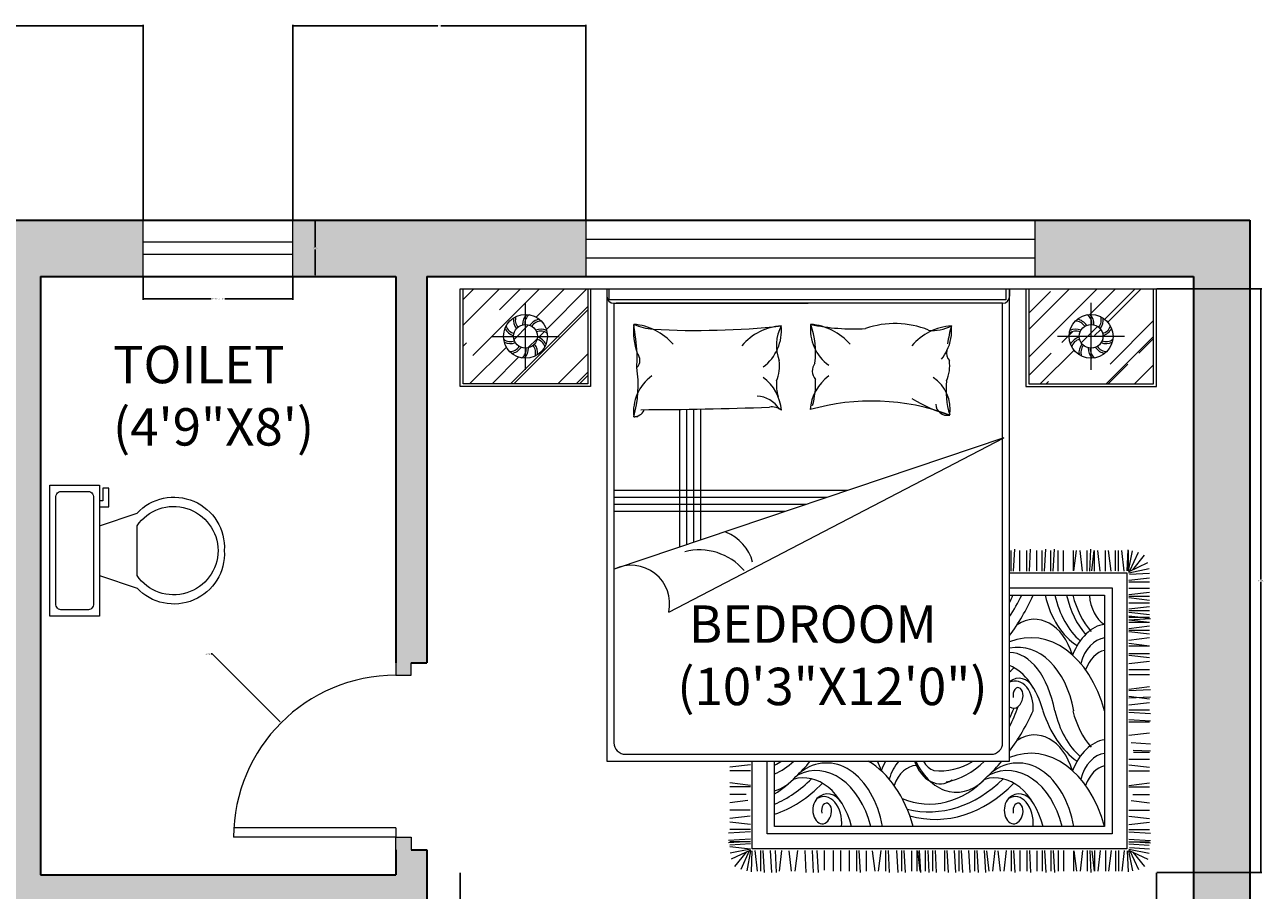
# Model space of a CAD drawing. Units: inches. Extents: x 2948 to 4025, y 2171 to 2966.
# Tile 5 of 6: x 3159 to 3358, y 2670 to 2809. Entities that reach past the tile are written whole.
import ezdxf

# ---------------------------------------------------------------- set-up
doc = ezdxf.new("R2010")
doc.units = ezdxf.units.IN
for name, color, linetype, lineweight in [('A-ANNO-DIMS', 2, 'Continuous', 18), ('A-AREA-IDEN', 7, 'Continuous', 18), ('A-DOOR', 3, 'Continuous', 18), ('A-FLOR-FIXT', 9, 'Continuous', 18), ('A-FURN', 8, 'Continuous', 18), ('A-GLAZ', 4, 'Continuous', 18), ('A-WALL', 7, 'Continuous', 35), ('A-WALL-PATT', 252, 'Continuous', 13)]:
    doc.layers.add(name, color=color, linetype=linetype, lineweight=lineweight)
doc.styles.get("Standard").update_dxf_attribs({"font": 'arial.ttf'})
doc.dimstyles.get("Standard").update_dxf_attribs({"dimtxt": 0.18, "dimasz": 0.18, "dimexe": 0.18, "dimexo": 0.0625, "dimgap": 0.09, "dimtad": 0, "dimtih": 1, "dimtoh": 1, "dimdec": 4, "dimzin": 0, "dimdsep": 46, "dimtxsty": 'Standard', "dimcen": 0.09, "dimadec": 0, "dimazin": 0, "dimtfac": 1, "dimtdec": 4, "dimtofl": 0, "dimtmove": 0, "dimatfit": 3, "dimfxl": 1, "dimtolj": 1, "dimtzin": 0, "dimarcsym": 0})

# ---------------------------------------------------------------- blocks, each defined once
blk = doc.blocks.new('A$C64B41DC1')
for p, q in [((0, 2.5079), (2.9903, 2.5079)), ((0, 2.0879), (0, 2.5079)), ((0.012, 2.4618), (0.0581, 2.5079)), ((0.012, 2.3515), (0.1684, 2.5079)), ((0.012, 2.0999), (0.012, 2.5079)), ((0.0543, 2.2213), (0.3409, 2.5079)), ((0.1689, 2.4179), (0.2589, 2.5079)), ((0.3265, 2.386), (0.4484, 2.5079)), ((0.3699, 2.3332), (0.5445, 2.5079)), ((0.548, 2.5079), (0.548, 2.0999)), ((0.56, 2.5079), (0.56, 2.0879)), ((0.6301, 2.5079), (0.6301, 0.4779)), ((0.6401, 2.461), (0.6401, 2.5079)), ((0.6401, 2.5079), (2.344, 2.5079)), ((2.344, 2.5079), (2.3601, 2.5079)), ((2.344, 2.5079), (2.344, 2.461)), ((2.3601, 2.5079), (2.3601, 2.4761)), ((2.3601, 0.4779), (2.3601, 2.5079)), ((2.4303, 2.5079), (2.4303, 2.0879)), ((2.4423, 2.5079), (2.4423, 2.0999)), ((2.4423, 2.3333), (2.6169, 2.5079)), ((2.4423, 2.2145), (2.7357, 2.5079)), ((2.705, 2.398), (2.8149, 2.5079)), ((2.7691, 2.3772), (2.8998, 2.5079)), ((2.7819, 2.3646), (2.9252, 2.5079)), ((2.9783, 2.0999), (2.9783, 2.5079)), ((2.9903, 2.0879), (2.9903, 2.5079)), ((0.2804, 2.1597), (0.2804, 2.4481)), ((2.344, 2.461), (0.6401, 2.461)), ((2.4423, 2.404), (2.5354, 2.4971)), ((2.7099, 2.1597), (2.7099, 2.4481)), ((0.2157, 2.0999), (0.548, 2.4322)), ((0.2299, 2.0999), (0.548, 2.418)), ((0.6601, 2.4461), (1.4951, 2.4461)), ((0.6601, 2.4461), (0.6601, 0.5579)), ((1.4951, 2.4461), (0.6697, 2.4461)), ((2.3301, 2.4461), (1.4951, 2.4461)), ((2.3301, 0.5579), (2.3301, 2.4461)), ((0.2311, 2.2906), (0.2937, 2.3532)), ((2.6674, 2.2756), (2.7382, 2.3464)), ((2.7914, 2.1846), (2.9783, 2.3715)), ((0.1362, 2.3039), (0.4246, 2.3039)), ((0.2905, 2.2539), (0.3304, 2.2938)), ((0.3405, 2.3039), (0.3605, 2.3238)), ((2.8541, 2.3039), (2.5657, 2.3039)), ((2.5849, 2.2779), (2.6158, 2.3088)), ((2.6158, 2.3088), (2.6313, 2.3243)), ((2.7249, 2.3076), (2.7512, 2.3339)), ((2.7746, 2.0999), (2.9783, 2.3036)), ((2.9144, 2.2312), (2.9783, 2.2951)), ((0.012, 2.261), (0.0275, 2.2765)), ((0.0404, 2.0999), (0.1982, 2.2578)), ((2.4918, 2.0999), (2.6366, 2.2447)), ((0.1365, 2.0999), (0.251, 2.2144)), ((0.4194, 2.0999), (0.548, 2.2285)), ((2.4423, 2.1353), (2.5382, 2.2312)), ((2.7831, 2.0999), (2.8678, 2.1846)), ((2.8962, 2.0999), (2.9783, 2.182)), ((0.4986, 2.0999), (0.548, 2.1493)), ((0.5127, 2.0999), (0.548, 2.1352)), ((0.56, 2.0879), (0, 2.0879)), ((0.548, 2.0999), (0.012, 2.0999)), ((2.4303, 2.0879), (2.9903, 2.0879)), ((2.4423, 2.0999), (2.9783, 2.0999)), ((2.5172, 2.0999), (2.5269, 2.1096)), ((0.9415, 1.9902), (0.9415, 1.3975)), ((0.9715, 1.9906), (0.9715, 1.4076)), ((1.0015, 1.991), (1.0015, 1.4177)), ((1.0315, 1.9916), (1.0315, 1.4279)), ((2.3349, 1.8678), (0.6613, 1.3029)), ((0.8956, 1.1191), (2.3349, 1.8678)), ((1.6636, 1.6412), (0.6601, 1.6412)), ((1.5748, 1.6112), (0.6601, 1.6112)), ((2.3665, 1.295), (2.3665, 1.3839)), ((2.377, 1.295), (2.3822, 1.3891)), ((2.4032, 1.295), (2.4032, 1.3839)), ((2.4346, 1.295), (2.4346, 1.3839)), ((2.4451, 1.295), (2.4503, 1.3891)), ((2.4774, 1.2957), (2.4774, 1.3837)), ((2.5, 1.295), (2.5, 1.3839)), ((2.5105, 1.295), (2.5157, 1.3891)), ((2.5367, 1.295), (2.5367, 1.3839)), ((2.5471, 1.295), (2.5524, 1.3891)), ((2.5681, 1.295), (2.5681, 1.3839)), ((2.5918, 1.295), (2.5918, 1.3839)), ((2.6346, 1.2957), (2.6346, 1.3837)), ((2.6362, 1.2957), (2.6467, 1.3839)), ((2.6729, 1.295), (2.6624, 1.3839)), ((2.6938, 1.295), (2.6938, 1.3839)), ((2.7043, 1.295), (2.7095, 1.3891)), ((2.7127, 1.2957), (2.7232, 1.3839)), ((2.7253, 1.295), (2.7253, 1.3839)), ((2.7494, 1.295), (2.7389, 1.3839)), ((2.7718, 1.295), (2.7718, 1.3839)), ((2.7959, 1.295), (2.7854, 1.3839)), ((2.8146, 1.2957), (2.8146, 1.3837)), ((2.8146, 1.2957), (2.8146, 1.3837)), ((2.8282, 1.295), (2.8282, 1.3839)), ((2.8282, 1.295), (2.8282, 1.3839)), ((2.8523, 1.295), (2.8418, 1.3839)), ((2.8523, 1.295), (2.8418, 1.3839)), ((2.8653, 1.2966), (2.8688, 1.3861)), ((2.8711, 1.2957), (2.8711, 1.3837)), ((2.8711, 1.2957), (2.8875, 1.3822)), ((2.8713, 1.2927), (2.954, 1.3315)), ((2.8765, 1.2958), (2.9132, 1.3758)), ((2.8893, 1.3011), (2.9394, 1.3636)), ((2.3601, 1.2873), (2.8639, 1.2873)), ((2.8639, 1.2873), (2.8639, 0.1018)), ((2.8717, 1.2884), (2.9588, 1.3058)), ((2.8744, 1.2817), (2.9603, 1.2869)), ((2.8716, 1.2565), (2.9605, 1.2669)), ((2.8723, 1.2489), (2.9603, 1.2489)), ((2.3601, 1.2233), (2.7999, 1.2233)), ((2.3601, 1.1913), (2.7679, 1.1912)), ((2.7679, 1.1912), (2.7679, 0.1978)), ((2.7999, 1.2233), (2.7999, 0.1658)), ((2.8716, 1.2212), (2.9605, 1.2212)), ((2.8716, 1.1947), (2.9605, 1.2052)), ((2.8716, 1.181), (2.9605, 1.1705)), ((2.8723, 1.1872), (2.9603, 1.1872)), ((2.8716, 1.1595), (2.9605, 1.1595)), ((2.8716, 1.133), (2.9605, 1.1435)), ((2.8716, 1.1193), (2.9605, 1.1088)), ((2.8723, 1.1255), (2.9603, 1.1255)), ((2.8716, 1.1035), (2.9605, 1.093)), ((2.8716, 1.0965), (2.9605, 1.0965)), ((2.8716, 1.086), (2.9657, 1.0913)), ((2.8716, 1.0756), (2.9605, 1.0756)), ((2.8723, 1.0858), (2.9605, 1.0753)), ((2.8716, 1.0491), (2.9605, 1.0596)), ((2.8716, 1.0354), (2.9605, 1.0249)), ((2.8723, 1.0416), (2.9603, 1.0416)), ((2.8723, 0.9987), (2.9605, 1.0092)), ((2.8723, 0.985), (2.9605, 0.9745)), ((2.8723, 0.9735), (2.9603, 0.9735)), ((2.8716, 0.9346), (2.9605, 0.9241)), ((2.8723, 0.9408), (2.9603, 0.9408)), ((2.8723, 0.8979), (2.9605, 0.9084)), ((2.8723, 0.8726), (2.9603, 0.8726)), ((2.8716, 0.7885), (2.9605, 0.799)), ((2.8723, 0.8505), (2.9603, 0.8505)), ((2.8716, 0.7818), (2.9657, 0.787)), ((2.8716, 0.7503), (2.9657, 0.7556)), ((2.8723, 0.7571), (2.9605, 0.7466)), ((2.8716, 0.7204), (2.9605, 0.7309)), ((2.8716, 0.6995), (2.9605, 0.6995)), ((2.8716, 0.689), (2.9657, 0.6838)), ((2.8716, 0.6576), (2.9657, 0.6523)), ((2.8716, 0.6471), (2.9605, 0.6471)), ((2.8716, 0.5903), (2.9605, 0.6007)), ((2.882, 0.5582), (2.9657, 0.5536)), ((0.7101, 0.5079), (2.2801, 0.5079)), ((2.8716, 0.4877), (2.9603, 0.4877)), ((2.8909, 0.5263), (2.9657, 0.5222)), ((2.8928, 0.5169), (2.9605, 0.5169)), ((0.6301, 0.4779), (2.3601, 0.4779)), ((1.2465, 0.4625), (1.1576, 0.452)), ((1.2465, 0.4365), (1.1577, 0.4365)), ((1.2542, 0.1018), (1.2542, 0.4779)), ((1.3182, 0.1658), (1.3182, 0.4779)), ((1.3502, 0.1978), (1.3502, 0.4779)), ((2.8716, 0.4625), (2.9605, 0.452)), ((2.8716, 0.4365), (2.9603, 0.4365)), ((1.2465, 0.3746), (1.1576, 0.3851)), ((2.8716, 0.3746), (2.9605, 0.3851)), ((1.2465, 0.3684), (1.1577, 0.3684)), ((1.2285, 0.3357), (1.1577, 0.3357)), ((2.8716, 0.3684), (2.9603, 0.3684)), ((2.8896, 0.3357), (2.9603, 0.3357)), ((1.2355, 0.3092), (1.1576, 0.3)), ((1.2457, 0.2676), (1.1577, 0.2676)), ((2.8723, 0.2676), (2.9603, 0.2676)), ((2.8826, 0.3092), (2.9605, 0.3)), ((1.2457, 0.2423), (1.1576, 0.2319)), ((1.2465, 0.2057), (1.1576, 0.2161)), ((2.8716, 0.2057), (2.9605, 0.2161)), ((2.8723, 0.2423), (2.9605, 0.2319)), ((1.2465, 0.1742), (1.1524, 0.169)), ((1.2465, 0.1847), (1.1576, 0.1847)), ((2.7999, 0.1658), (1.3182, 0.1658)), ((2.7679, 0.1978), (1.3502, 0.1978)), ((2.8716, 0.1847), (2.9605, 0.1847)), ((2.8716, 0.1742), (2.9657, 0.169)), ((1.2465, 0.1428), (1.1524, 0.1376)), ((1.2465, 0.1334), (1.1524, 0.1281)), ((1.2465, 0.1323), (1.1576, 0.1323)), ((1.2465, 0.1323), (1.1576, 0.1323)), ((1.2465, 0.1), (1.1576, 0.1105)), ((1.2465, 0.1229), (1.1588, 0.1168)), ((2.8716, 0.1428), (2.9657, 0.1376)), ((2.8716, 0.1334), (2.9657, 0.1281)), ((2.8716, 0.1323), (2.9605, 0.1323)), ((2.8716, 0.1229), (2.9593, 0.1168)), ((2.8744, 0.1074), (2.9603, 0.1022)), ((1.2464, 0.1007), (1.1592, 0.0833)), ((1.2468, 0.0964), (1.1641, 0.0576)), ((1.2288, 0.088), (1.1787, 0.0255)), ((1.2415, 0.0933), (1.2049, 0.0133)), ((1.247, 0.0934), (1.2306, 0.0069)), ((1.2527, 0.0925), (1.2493, 0.003)), ((2.8639, 0.1018), (1.2542, 0.1018)), ((1.2658, 0.0941), (1.2762, 0.0052)), ((1.2899, 0.0941), (1.2899, 0.0052)), ((1.2999, 0.0941), (1.3051, 0)), ((1.3313, 0.0941), (1.3365, 0)), ((1.3523, 0.0941), (1.3575, 0)), ((1.3804, 0.0941), (1.3699, 0.0052)), ((1.4119, 0.0934), (1.4223, 0.0052)), ((1.4485, 0.0941), (1.438, 0.0052)), ((1.48, 0.0941), (1.4852, 0)), ((1.5114, 0.0941), (1.5166, 0)), ((1.5323, 0.0941), (1.5376, 0)), ((1.5638, 0.0941), (1.5638, 0.0105)), ((1.6021, 0.0941), (1.6021, 0.0052)), ((1.6336, 0.0941), (1.6336, 0.0052)), ((1.6702, 0.0941), (1.6702, 0.0052)), ((1.7017, 0.0941), (1.7017, 0.0052)), ((1.7122, 0.0941), (1.7174, 0)), ((1.7445, 0.0934), (1.7445, 0.0054)), ((1.7698, 0.0934), (1.7803, 0.0052)), ((1.8065, 0.0941), (1.796, 0.0052)), ((1.8274, 0.0941), (1.8274, 0.0052)), ((1.8379, 0.0941), (1.8431, 0)), ((1.8746, 0.0941), (1.8798, 0)), ((1.8955, 0.0941), (1.8955, 0.0052)), ((1.906, 0.0941), (1.9113, 0)), ((1.9384, 0.0934), (1.9384, 0.0054)), ((1.9609, 0.0941), (1.9609, 0.0052)), ((1.9636, 0.0934), (1.9741, 0.0052)), ((1.9714, 0.0941), (1.9766, 0)), ((1.9976, 0.0941), (1.9976, 0.0052)), ((2.0081, 0.0941), (2.0133, 0)), ((2.029, 0.0941), (2.029, 0.0052)), ((2.0395, 0.0941), (2.0447, 0)), ((2.0797, 0.0941), (2.0797, 0.0052)), ((2.0902, 0.0941), (2.0954, 0)), ((2.1216, 0.0941), (2.1269, 0)), ((2.1412, 0.0941), (2.1412, 0.0052)), ((2.1517, 0.0941), (2.1569, 0)), ((2.1831, 0.0941), (2.1884, 0)), ((2.2093, 0.0941), (2.2093, 0.0052)), ((2.2198, 0.0941), (2.225, 0)), ((2.2512, 0.0941), (2.2565, 0)), ((2.2603, 0.0934), (2.2707, 0.0052)), ((2.2969, 0.0941), (2.2864, 0.0052)), ((2.3089, 0.0934), (2.3193, 0.0052)), ((2.3455, 0.0941), (2.3351, 0.0052)), ((2.3665, 0.0941), (2.3665, 0.0052)), ((2.377, 0.0941), (2.3822, 0)), ((2.4032, 0.0941), (2.4032, 0.0052)), ((2.4346, 0.0941), (2.4346, 0.0052)), ((2.4451, 0.0941), (2.4503, 0)), ((2.4774, 0.0934), (2.4774, 0.0054)), ((2.5, 0.0941), (2.5, 0.0052)), ((2.5105, 0.0941), (2.5157, 0)), ((2.5367, 0.0941), (2.5367, 0.0052)), ((2.5471, 0.0941), (2.5524, 0)), ((2.5681, 0.0941), (2.5681, 0.0052)), ((2.5918, 0.0941), (2.5918, 0.0052)), ((2.6346, 0.0934), (2.6346, 0.0054)), ((2.6362, 0.0934), (2.6467, 0.0052)), ((2.6729, 0.0941), (2.6624, 0.0052)), ((2.6938, 0.0941), (2.6938, 0.0052)), ((2.7043, 0.0941), (2.7095, 0)), ((2.7127, 0.0934), (2.7232, 0.0052)), ((2.7253, 0.0941), (2.7253, 0.0052)), ((2.7494, 0.0941), (2.7389, 0.0052)), ((2.7718, 0.0941), (2.7718, 0.0052)), ((2.7959, 0.0941), (2.7854, 0.0052)), ((2.8146, 0.0934), (2.8146, 0.0054)), ((2.8282, 0.0941), (2.8282, 0.0052)), ((2.8523, 0.0941), (2.8418, 0.0052)), ((2.8653, 0.0925), (2.8688, 0.003)), ((2.8711, 0.0934), (2.8875, 0.0069)), ((2.8713, 0.0964), (2.954, 0.0576)), ((2.8717, 0.1007), (2.9588, 0.0833)), ((2.8765, 0.0933), (2.9132, 0.0133)), ((2.8893, 0.088), (2.9394, 0.0255))]:
    blk.add_line(p, q)
at = {"ltscale": 10}
for p, q in [((1.4859, 1.5812), (0.6601, 1.5812)), ((1.397, 1.5512), (0.6601, 1.5512))]:
    blk.add_line(p, q, dxfattribs=at)
for centre, radius in [((0.2804, 2.3039), 0.0942), ((2.7099, 2.3039), 0.0942), ((0.2804, 2.3039), 0.051), ((2.7099, 2.3039), 0.051)]:
    blk.add_circle(centre, radius)
for centre, radius, start, end in [((0.6601, 2.4761), 0.03, 180, 270), ((2.3301, 2.4761), 0.03, 270, 0), ((0.3286, 2.3561), 0.0605, 136.17, 182.4897), ((0.3231, 2.3585), 0.0462, 124.3002, 184.538), ((2.6672, 2.3585), 0.0462, 355.462, 55.6998), ((2.6617, 2.3561), 0.0605, 357.5103, 43.83), ((0.2417, 2.3614), 0.0462, 196.3002, 256.538), ((0.2887, 2.3745), 0.0605, 172.17, 218.4897), ((0.2828, 2.3731), 0.0462, 160.3002, 220.538), ((0.3501, 2.3178), 0.0605, 100.17, 146.4897), ((0.347, 2.323), 0.0462, 88.3002, 148.538), ((1.0526, 2.3302), 0.3085, 175.3048, 198.6942), ((-0.8702, 2.0941), 1.6364, 4.8098, 9.1892), ((0.8579, 2.6278), 0.2948, 247.5179, 264.267), ((0.728, 2.111), 0.245, 40.4189, 85.9871), ((1.0164, 5.7096), 3.3803, 266.8134, 276.1602), ((1.3963, 2.1044), 0.245, 94.0129, 139.5811), ((1.1858, 2.3288), 0.1943, 306.5711, 5.89), ((1.5348, 2.2652), 0.1767, 151.7736, 201.6983), ((1.6986, 2.3355), 0.1943, 174.11, 233.4289), ((1.1481, 2.2311), 0.3783, 353.4947, 19.1867), ((1.6871, 3.192), 0.8561, 257.7438, 273.6284), ((1.4882, 2.111), 0.245, 40.4189, 85.9871), ((1.8674, 1.9709), 0.3878, 68.2026, 108.9817), ((2.1269, 2.1044), 0.245, 94.0129, 139.5811), ((2.0342, 2.4856), 0.1563, 261.5958, 298.9092), ((1.9165, 2.3288), 0.1943, 333.7371, 5.89), ((2.6058, 2.2028), 0.517, 163.6046, 172.3273), ((2.6433, 2.323), 0.0462, 31.462, 91.6998), ((2.6402, 2.3178), 0.0605, 33.5103, 79.83), ((2.7075, 2.3731), 0.0462, 319.462, 19.6998), ((2.7016, 2.3745), 0.0605, 321.5103, 7.83), ((2.7486, 2.3614), 0.0462, 283.462, 343.6998), ((0.2153, 2.3276), 0.0462, 232.3002, 292.538), ((0.2457, 2.3659), 0.0605, 208.17, 254.4897), ((0.3449, 2.2742), 0.0605, 64.17, 110.4897), ((0.3455, 2.2802), 0.0462, 52.3002, 112.538), ((0.3191, 2.2464), 0.0462, 16.3002, 76.538), ((0.3151, 2.2419), 0.0605, 28.17, 74.4897), ((2.6448, 2.2802), 0.0462, 67.462, 127.6998), ((2.6454, 2.2742), 0.0605, 69.5103, 115.83), ((2.6752, 2.2419), 0.0605, 105.5103, 151.83), ((2.6712, 2.2464), 0.0462, 103.462, 163.6998), ((2.775, 2.3276), 0.0462, 247.462, 307.6998), ((2.7446, 2.3659), 0.0605, 285.5103, 331.83), ((0.2158, 2.3336), 0.0605, 244.17, 290.4897), ((0.2138, 2.2848), 0.0462, 268.3002, 328.538), ((0.2107, 2.29), 0.0605, 280.17, 326.4897), ((0.2377, 2.2493), 0.0462, 304.3002, 4.538), ((0.2322, 2.2517), 0.0605, 316.17, 2.4897), ((0.2779, 2.2347), 0.0462, 340.3002, 40.538), ((0.272, 2.2333), 0.0605, 352.17, 38.4897), ((1.9165, 2.3288), 0.1943, 320.9404, 333.7371), ((2.1347, 2.2313), 0.0459, 165.3506, 223.2684), ((2.7182, 2.2333), 0.0605, 141.5103, 187.83), ((2.7123, 2.2347), 0.0462, 139.462, 199.6998), ((2.7581, 2.2517), 0.0605, 177.5103, 223.83), ((2.7526, 2.2493), 0.0462, 175.462, 235.6998), ((2.7796, 2.29), 0.0605, 213.5103, 259.83), ((2.7765, 2.2848), 0.0462, 211.462, 271.6998), ((2.7744, 2.3336), 0.0605, 249.5103, 295.83), ((0.7274, 2.2013), 0.0446, 314.4736, 42.1713), ((-1.6008, 2.277), 2.3618, 357.3905, 358.8876), ((1.204, 2.1778), 0.1681, 337.017, 7.5368), ((1.5671, 2.1546), 0.0547, 142.0833, 220.902), ((1.9346, 2.1778), 0.1681, 337.017, 7.5368), ((0.9385, 1.978), 0.1943, 126.5711, 185.89), ((0.2688, 2.0945), 0.4956, 344.0243, 8.7071), ((1.7059, 1.9714), 0.204, 127.1197, 175.09), ((1.1858, 1.9714), 0.1943, 4.3181, 53.4289), ((1.5415, 2.0969), 0.1834, 175.2233, 196.23), ((1.1965, 2.0983), 0.3299, 343.7954, 3.5554), ((1.9394, 1.991), 0.1651, 351.2621, 55.7572), ((2.4617, 2.0719), 0.3745, 173.8296, 196.4356), ((1.2687, 1.9248), 0.1223, 33.628, 86.4744), ((1.7676, 1.0629), 0.9631, 69.6507, 105.9631), ((2.2748, 2.5795), 0.6373, 238.3499, 254.3137), ((0.7417, 2.0149), 0.057, 273.4709, 328.5412), ((0.7246, 18.8439), 16.8552, 270.17399, 272.05214), ((1.3401, 1.9404), 0.0603, 49.0991, 101.3702), ((2.0911, 2.0123), 0.0478, 179.7727, 283.8018), ((0.728, 2.2025), 0.245, 274.0129, 278.3417), ((1.0747, 1.2871), 0.1871, 14.1863, 69.1212), ((1.0274, 1.1334), 0.2527, 40.629, 104.3712), ((0.7347, 1.1553), 0.1649, 347.3109, 116.4454), ((0.7101, 0.5579), 0.05, 180, 270), ((2.2801, 0.5579), 0.05, 270, 0)]:
    blk.add_arc(centre, radius, start, end)
for centre, major_axis, ratio, start_param, end_param in [((1.9938, 1.6262), (0, -0.7531), 0.68, 0.797284, 0.954936), ((2.0643, 1.466), (0, -0.5322), 0.68, 7.239912, 7.311536), ((1.9052, 1.7397), (0, -0.9842), 0.68, 0.74745, 0.979724), ((2.7455, 1.3081), (0, 0.3614), 0.68, 1.900046, 2.742661), ((2.7868, 1.3081), (0, 0.3614), 0.68, 1.900046, 2.614747), ((2.8372, 1.3081), (0, 0.3614), 0.68, 1.900046, 2.479658), ((2.8607, 1.3211), (0, 0.3614), 0.68, 1.938265, 2.479658), ((2.8057, 1.2079), (0, -0.1524), 0.68, 4.821745, 5.895886), ((2.4665, 0.8216), (0, -0.2664), 0.68, 2.006169, 3.565187), ((2.7862, 0.8069), (0, -0.2615), 0.68, 3.244645, 4.205018), ((2.4513, 0.5069), (0, 0.502), 0.68, 5.095327, 6.553458), ((2.396, 0.6032), (0, 0.3641), 0.68, -1.3172, 0.145284), ((2.7784, 0.8289), (0, -0.1802), 0.68, 3.227058, 4.318474), ((2.3507, 0.5642), (0.0073, 0.3819), 0.56205, -1.21172, -0.009991), ((2.7821, 0.7971), (0, -0.1589), 0.68, 3.272942, 4.229533), ((2.2964, 0.5771), (0, -0.3263), 0.68, 1.938944, 2.850232), ((2.0403, 1.6015), (0, -0.8763), 0.68, 6.849801, 6.887077), ((2.4005, 0.7132), (0, -0.1214), 0.68, 2.284368, 3.652258), ((2.3834, 0.7081), (0, 0.1147), 0.68, 4.593909, 6.585576), ((2.3774, 0.7653), (0, -0.0593), 0.68, 5.841311, 7.755362), ((2.3961, 0.7628), (0, -0.0317), 0.68, 1.462497, 5.046281), ((1.9938, 1.1295), (-0.0678, 0.7439), 0.610498, 3.917146, 4.063997), ((2.0643, 0.9693), (0, -0.5322), 0.68, 7.239912, 7.336618), ((1.9052, 1.243), (0, -0.9842), 0.68, 0.74745, 0.979724), ((2.7455, 0.8114), (-0.0599, 0.3735), 0.695517, 1.775813, 2.548612), ((2.7868, 0.8114), (0, 0.3614), 0.68, 1.900046, 2.614747), ((2.8607, 0.8243), (0, 0.3614), 0.68, 1.938265, 2.479658), ((2.4665, 0.3249), (0, -0.2664), 0.68, 2.006169, 3.565187), ((2.4513, 0.0102), (0, 0.502), 0.68, 5.095327, 6.553458), ((2.7862, 0.3102), (0, -0.2615), 0.68, 3.244645, 4.205018), ((1.5283, 0.0674), (0, -0.3703), 0.68, 1.930561, 3.464283), ((1.5736, 0.1065), (0, 0.3641), 0.68, -1.3172, 0.476403), ((2.3507, 0.0674), (0, -0.3703), 0.68, 1.930561, 3.464283), ((2.396, 0.1065), (0, 0.3641), 0.68, -1.3172, 0.476403), ((2.7784, 0.3322), (0, -0.1802), 0.68, 3.227058, 4.318474), ((1.242, 0.9693), (0, -0.5322), 0.68, 6.586764, 6.677612), ((1.1714, 1.1295), (-0.1157, 0.7241), 0.59432, 3.291697, 3.50733), ((1.474, 0.0804), (0, -0.3263), 0.68, 1.938944, 3.339184), ((1.0828, 1.243), (0, -0.9842), 0.68, 0.565948, 0.680366), ((1.6289, 0.0102), (0, 0.502), 0.68, 6.655152, 6.661293), ((1.6289, 0.0102), (0, 0.502), 0.68, 5.095327, 5.911219), ((1.6442, 0.3249), (0, -0.2664), 0.68, 2.006169, 2.182797), ((1.9638, 0.3102), (0, -0.2615), 0.68, 4.015924, 4.205018), ((1.956, 0.3322), (0, -0.1802), 0.68, 3.770744, 4.318474), ((1.9597, 0.3004), (0, -0.1589), 0.68, 3.14258, 4.229533), ((2.0606, 0.5616), (0, -0.1803), 0.68, 5.194792, 5.929328), ((2.0606, 0.5616), (0, -0.1803), 0.68, 5.194792, 6.723255), ((2.1315, 0.6603), (0, -0.3155), 0.68, 5.328638, 6.949396), ((2.0549, 0.5656), (0, -0.1303), 0.68, 5.450951, 6.054641), ((2.0643, 0.9693), (0, -0.5322), 0.68, 6.20013, 6.677612), ((1.9938, 1.1295), (-0.0678, 0.7439), 0.610498, 3.199135, 3.592282), ((2.2964, 0.0804), (0, -0.3263), 0.68, 1.938944, 3.339184), ((1.9052, 1.243), (0, -0.9842), 0.68, 0.565948, 0.680366), ((2.4513, 0.0102), (0, 0.502), 0.68, 6.655152, 6.661293), ((2.7821, 0.3004), (0, -0.1589), 0.68, 3.272942, 4.229533), ((1.1933, 0.9181), (0, -0.624), 0.68, 0.378672, 0.625379), ((1.3091, 0.6603), (0, -0.3155), 0.68, 6.475719, 6.949396), ((1.1911, 1.1066), (0, 0.8458), 0.68, 3.421828, 3.728616), ((1.2179, 1.1047), (0, -0.8763), 0.68, 6.507006, 6.887077), ((2.0157, 0.9181), (0, -0.624), 0.68, -0.280078, 0.625379), ((2.0135, 1.1066), (0, 0.8458), 0.68, 2.978727, 3.728616), ((2.0403, 1.1047), (0, -0.8763), 0.68, 6.099302, 6.887077), ((1.5781, 0.2165), (0, -0.1214), 0.68, 2.284368, 3.726131), ((1.561, 0.2114), (0, 0.1147), 0.68, 4.593909, 6.647252), ((2.4005, 0.2165), (0, -0.1214), 0.68, 2.284368, 3.726131), ((2.3834, 0.2114), (0, 0.1147), 0.68, 4.593909, 6.647252), ((1.555, 0.2685), (0, -0.0593), 0.68, 3.732151, 7.755362), ((1.5737, 0.2661), (0, -0.0317), 0.68, 1.462497, 5.046281), ((2.3774, 0.2685), (0, -0.0593), 0.68, 3.732151, 7.755362), ((2.3961, 0.2661), (0, -0.0317), 0.68, 1.462497, 5.046281)]:
    blk.add_ellipse(centre, major_axis=major_axis, ratio=ratio, start_param=start_param, end_param=end_param)
blk = doc.blocks.new('*U8')
for p, q in [((9.5, -6), (9.5, -2)), ((-10, -8.5), (-8, -8.5)), ((-10, -9.5), (-10, -8.5)), ((-7, -9.5), (-10, -9.5)), ((-8, -8.5), (-8, -8)), ((-7, -8), (-7, -9.5)), ((-4, -8), (-6, -14)), ((4, -8), (6, -14)), ((4, -14), (-4, -14))]:
    blk.add_line(p, q)
blk.add_lwpolyline([(10.5, -8), (10.5, 0), (-10.5, 0), (-10.5, -8)], close=True)
for points in [[(8.5, -1), (-8.5, -1)], [(-9.5, -2), (-9.5, -6)], [(-8.5, -7), (8.5, -7)]]:
    blk.add_lwpolyline(points)
for centre, radius, start, end in [((-8.625, -1.875), 0.8839, 81.8699, 188.1301), ((8.625, -1.875), 0.8839, 351.8699, 98.1301), ((-8.625, -6.125), 0.8839, 171.869898, 278.1301), ((8.625, -6.125), 0.8839, 261.8699, 8.1301), ((-0.4772, -19.9188), 8.0953, 133.01722, 273.38), ((0.0374, -19.8731), 7.127, 124.50543, 269.7), ((-0.0373, -19.8731), 7.127, 270.3, 55.4946), ((0.4773, -19.9188), 8.0953, 266.62, 46.9828)]:
    blk.add_arc(centre, radius, start, end)
blk = doc.blocks.new('DOOR-SWING-26IN')
for p, q in [((26, 30), (26, 28)), ((28.5, 28), (28.5, 30)), ((26, 28), (28.5, 28)), ((26, 2), (0, 2)), ((26, 3.5), (0.04, 3.5)), ((26, 3.5), (26, 2)), ((26, 0), (26, 2)), ((26, 2), (28.5, 2)), ((28.5, 2), (28.5, 0))]:
    blk.add_line(p, q)
blk.add_arc((26, 2), 26, 90, 180)
blk = doc.blocks.new('WIN-72IN')
for p, q in [((0, 0), (0, 9)), ((72, 0), (72, 9)), ((72, 6), (0, 6)), ((72, 3), (0, 3))]:
    blk.add_line(p, q)
blk = doc.blocks.new('WIN-24IN')
for p, q in [((0, 0), (0, 9)), ((24, 0), (24, 9)), ((24, 5.5), (0, 5.5)), ((24, 3.5), (0, 3.5))]:
    blk.add_line(p, q)
blk = doc.blocks.new('*D23')
at = {"layer": 'A-ANNO-DIMS', "color": 0, "lineweight": -2, "transparency": 16777216}
for p, q in [((3178.01, 2768.92), (3178.01, 2765.21)), ((3202.01, 2768.92), (3202.01, 2765.21)), ((3178.19, 2765.39), (3188.9, 2765.39)), ((3201.83, 2765.39), (3191.13, 2765.39))]:
    blk.add_line(p, q, dxfattribs=at)
at = {"layer": 'A-ANNO-DIMS', "color": 0, "transparency": 16777216}
for points in [[(3178.19, 2765.42), (3178.19, 2765.36), (3178.01, 2765.39)], [(3201.83, 2765.42), (3201.83, 2765.36), (3202.01, 2765.39)]]:
    blk.add_solid(points, dxfattribs=at)
at = {"layer": 'Defpoints', "color": 0, "transparency": 16777216}
for p in [(3178.01, 2768.99), (3202.01, 2768.99), (3202.01, 2765.39)]:
    blk.add_point(p, dxfattribs=at)
at = {"layer": 'A-ANNO-DIMS', "color": 0, "transparency": 16777216, "insert": (3190.01, 2765.39), "char_height": 0.18, "attachment_point": 5}
blk.add_mtext('\\A1;WINDOW 24 TYP.', dxfattribs=at)
blk = doc.blocks.new('*D24')
at = {"layer": 'A-ANNO-DIMS', "color": 0, "lineweight": -2, "transparency": 16777216}
for p, q in [((3202.08, 2777.99), (3205.79, 2777.99)), ((3205.61, 2777.81), (3205.61, 2773.67)), ((3205.61, 2769.17), (3205.61, 2773.3)), ((3202.08, 2768.99), (3205.79, 2768.99))]:
    blk.add_line(p, q, dxfattribs=at)
at = {"layer": 'A-ANNO-DIMS', "color": 0, "transparency": 16777216}
for points in [[(3205.58, 2777.81), (3205.64, 2777.81), (3205.61, 2777.99)], [(3205.58, 2769.17), (3205.64, 2769.17), (3205.61, 2768.99)]]:
    blk.add_solid(points, dxfattribs=at)
at = {"layer": 'Defpoints', "color": 0, "transparency": 16777216}
for p in [(3202.01, 2777.99), (3205.61, 2777.99), (3202.01, 2768.99)]:
    blk.add_point(p, dxfattribs=at)
at = {"layer": 'A-ANNO-DIMS', "color": 0, "transparency": 16777216, "insert": (3205.61, 2773.49), "char_height": 0.18, "attachment_point": 5}
blk.add_mtext('\\A1;9 TYP.', dxfattribs=at)
blk = doc.blocks.new('*D27')
at = {"layer": 'A-ANNO-DIMS', "color": 0, "lineweight": -2, "transparency": 16777216}
for p, q in [((3228.87, 2673.27), (3228.87, 2656.41)), ((3340.53, 2673.27), (3340.53, 2656.41)), ((3229.05, 2656.59), (3283.31, 2656.59)), ((3340.35, 2656.59), (3286.08, 2656.59))]:
    blk.add_line(p, q, dxfattribs=at)
at = {"layer": 'A-ANNO-DIMS', "color": 0, "transparency": 16777216}
for points in [[(3229.05, 2656.62), (3229.05, 2656.56), (3228.87, 2656.59)], [(3340.35, 2656.62), (3340.35, 2656.56), (3340.53, 2656.59)]]:
    blk.add_solid(points, dxfattribs=at)
at = {"layer": 'Defpoints', "color": 0, "transparency": 16777216}
for p in [(3228.87, 2673.34), (3340.53, 2673.34), (3340.53, 2656.59)]:
    blk.add_point(p, dxfattribs=at)
at = {"layer": 'A-ANNO-DIMS', "color": 0, "transparency": 16777216, "insert": (3284.7, 2656.59), "char_height": 0.18, "attachment_point": 5}
blk.add_mtext('\\A1;BED GROUP 112 TYP.', dxfattribs=at)
blk = doc.blocks.new('*D28')
at = {"layer": 'A-ANNO-DIMS', "color": 0, "lineweight": -2, "transparency": 16777216}
for p, q in [((3340.59, 2766.99), (3357.46, 2766.99)), ((3357.28, 2766.81), (3357.28, 2720.34)), ((3357.28, 2673.52), (3357.28, 2719.98)), ((3340.59, 2673.34), (3357.46, 2673.34))]:
    blk.add_line(p, q, dxfattribs=at)
at = {"layer": 'A-ANNO-DIMS', "color": 0, "transparency": 16777216}
for points in [[(3357.25, 2766.81), (3357.31, 2766.81), (3357.28, 2766.99)], [(3357.25, 2673.52), (3357.31, 2673.52), (3357.28, 2673.34)]]:
    blk.add_solid(points, dxfattribs=at)
at = {"layer": 'Defpoints', "color": 0, "transparency": 16777216}
for p in [(3340.53, 2766.99), (3357.28, 2766.99), (3340.53, 2673.34)]:
    blk.add_point(p, dxfattribs=at)
at = {"layer": 'A-ANNO-DIMS', "color": 0, "transparency": 16777216, "insert": (3357.28, 2720.16), "char_height": 0.18, "attachment_point": 5}
blk.add_mtext('\\A1;94 TYP.', dxfattribs=at)
blk = doc.blocks.new('*D38')
at = {"layer": 'A-ANNO-DIMS', "color": 0, "lineweight": -2, "transparency": 16777216}
for p, q in [((2979.45, 2777.99), (2948.13, 2777.99)), ((2948.31, 2777.81), (2948.31, 2507.17)), ((2948.31, 2236.17), (2948.31, 2506.8)), ((3217.45, 2235.99), (2948.13, 2235.99))]:
    blk.add_line(p, q, dxfattribs=at)
at = {"layer": 'A-ANNO-DIMS', "color": 0, "transparency": 16777216}
for points in [[(2948.28, 2777.81), (2948.34, 2777.81), (2948.31, 2777.99)], [(2948.28, 2236.17), (2948.34, 2236.17), (2948.31, 2235.99)]]:
    blk.add_solid(points, dxfattribs=at)
at = {"layer": 'Defpoints', "color": 0, "transparency": 16777216}
for p in [(2948.31, 2777.99), (2979.51, 2777.99), (3217.51, 2235.99)]:
    blk.add_point(p, dxfattribs=at)
at = {"layer": 'A-ANNO-DIMS', "color": 0, "transparency": 16777216, "insert": (2948.31, 2506.99), "char_height": 0.18, "attachment_point": 5}
blk.add_mtext('\\A1;542', dxfattribs=at)
blk = doc.blocks.new('*D40')
at = {"layer": 'A-ANNO-DIMS', "color": 0, "lineweight": -2, "transparency": 16777216}
for p, q in [((3108.51, 2778.05), (3108.51, 2809.37)), ((3108.69, 2809.19), (3142.94, 2809.19)), ((3177.83, 2809.19), (3143.59, 2809.19)), ((3178.01, 2778.05), (3178.01, 2809.37))]:
    blk.add_line(p, q, dxfattribs=at)
at = {"layer": 'A-ANNO-DIMS', "color": 0, "transparency": 16777216}
for points in [[(3108.69, 2809.22), (3108.69, 2809.16), (3108.51, 2809.19)], [(3177.83, 2809.22), (3177.83, 2809.16), (3178.01, 2809.19)]]:
    blk.add_solid(points, dxfattribs=at)
at = {"layer": 'Defpoints', "color": 0, "transparency": 16777216}
for p in [(3178.01, 2809.19), (3108.51, 2777.99), (3178.01, 2777.99)]:
    blk.add_point(p, dxfattribs=at)
at = {"layer": 'A-ANNO-DIMS', "color": 0, "transparency": 16777216, "insert": (3143.26, 2809.19), "char_height": 0.18, "attachment_point": 5}
blk.add_mtext('\\A1;69.5', dxfattribs=at)
blk = doc.blocks.new('*D41')
at = {"layer": 'A-ANNO-DIMS', "color": 0, "lineweight": -2, "transparency": 16777216}
for p, q in [((3202.01, 2778.05), (3202.01, 2809.37)), ((3202.19, 2809.19), (3225.29, 2809.19)), ((3248.83, 2809.19), (3225.74, 2809.19)), ((3249.01, 2778.05), (3249.01, 2809.37))]:
    blk.add_line(p, q, dxfattribs=at)
at = {"layer": 'A-ANNO-DIMS', "color": 0, "transparency": 16777216}
for points in [[(3202.19, 2809.22), (3202.19, 2809.16), (3202.01, 2809.19)], [(3248.83, 2809.22), (3248.83, 2809.16), (3249.01, 2809.19)]]:
    blk.add_solid(points, dxfattribs=at)
at = {"layer": 'Defpoints', "color": 0, "transparency": 16777216}
for p in [(3249.01, 2809.19), (3202.01, 2777.99), (3249.01, 2777.99)]:
    blk.add_point(p, dxfattribs=at)
at = {"layer": 'A-ANNO-DIMS', "color": 0, "transparency": 16777216, "insert": (3225.51, 2809.19), "char_height": 0.18, "attachment_point": 5}
blk.add_mtext('\\A1;47', dxfattribs=at)
blk = doc.blocks.new('*D69')
at = {"layer": 'A-ANNO-DIMS', "color": 0, "lineweight": -2, "transparency": 16777216}
for p, q in [((3188.92, 2708.4), (3189.1, 2708.4)), ((3189.1, 2708.4), (3200, 2697.5)), ((3218.42, 2678.99), (3218.6, 2678.99)), ((3218.51, 2678.9), (3218.51, 2679.08))]:
    blk.add_line(p, q, dxfattribs=at)
at = {"layer": 'A-ANNO-DIMS', "color": 0, "transparency": 16777216}
blk.add_solid([(3200.02, 2697.52), (3199.98, 2697.48), (3200.13, 2697.37)], dxfattribs=at)
at = {"layer": 'Defpoints', "color": 0, "transparency": 16777216}
for p in [(3200.13, 2697.37), (3218.51, 2678.99)]:
    blk.add_point(p, dxfattribs=at)
at = {"layer": 'A-ANNO-DIMS', "color": 0, "transparency": 16777216, "insert": (3188.42, 2708.4), "char_height": 0.18, "attachment_point": 5}
blk.add_mtext('\\A1;2X R26', dxfattribs=at)

msp = doc.modelspace()

# ---------------------------------------------------------------- hatches: boundary and pattern name
at = {"layer": 'A-WALL-PATT'}
h = msp.add_hatch(color=256, dxfattribs=at)
h.dxf.hatch_style = 1
h.paths.add_polyline_path([(3178.0136, 2777.9862), (3108.5136, 2777.9862), (3108.5136, 2768.9862), (3156.5136, 2768.9862), (3156.5136, 2624.9862), (3132.5136, 2624.9862), (3130.5136, 2624.9862), (3130.5136, 2622.4862), (3132.5136, 2622.4862), (3132.5136, 2619.9862), (3161.5136, 2619.9862), (3161.5136, 2667.9862), (3218.5136, 2667.9862), (3218.5136, 2660.9862), (3218.5136, 2658.9862), (3221.0136, 2658.9862), (3221.0136, 2660.9862), (3223.5136, 2660.9862), (3223.5136, 2676.9862), (3221.0136, 2676.9862), (3221.0136, 2678.9862), (3218.5136, 2678.9862), (3218.5136, 2676.9862), (3218.5136, 2672.9862), (3161.5136, 2672.9862), (3161.5136, 2768.9862), (3178.0136, 2768.9862)])
h = msp.add_hatch(color=256, dxfattribs=at)
h.dxf.hatch_style = 1
h.paths.add_polyline_path([(3249.0136, 2777.9862), (3202.0136, 2777.9862), (3202.0136, 2768.9862), (3218.5136, 2768.9862), (3218.5136, 2706.9862), (3218.5136, 2704.9862), (3221.0136, 2704.9862), (3221.0136, 2706.9862), (3223.5136, 2706.9862), (3223.5136, 2768.9862), (3249.0136, 2768.9862)])
h = msp.add_hatch(color=256, dxfattribs=at)
h.dxf.hatch_style = 1
h.paths.add_polyline_path([(3355.5136, 2777.9862), (3321.0136, 2777.9862), (3321.0136, 2768.9862), (3346.5136, 2768.9862), (3346.5136, 2624.9862), (3221.0136, 2624.9862), (3221.0136, 2626.9862), (3218.5136, 2626.9862), (3218.5136, 2624.9862), (3218.5136, 2619.9862), (3346.5136, 2619.9862), (3346.5136, 2517.9862), (3355.5136, 2517.9862)])

# ---------------------------------------------------------------- linework, layer by layer
at = {"layer": 'A-WALL'}
for p, q in [((2979.5136, 2777.9862), (3355.5136, 2777.9862)), ((3355.5136, 2777.9862), (3355.5136, 2235.9862)), ((3161.5136, 2768.9862), (3161.5136, 2672.9862)), ((3161.5136, 2768.9862), (3218.5136, 2768.9862)), ((3218.5136, 2768.9862), (3218.5136, 2706.9862)), ((3223.5136, 2768.9862), (3223.5136, 2706.9862)), ((3223.5136, 2768.9862), (3346.5136, 2768.9862)), ((3346.5136, 2768.9862), (3346.5136, 2624.9862)), ((3221.0136, 2706.9862), (3223.5136, 2706.9862)), ((3218.5136, 2676.9862), (3218.5136, 2672.9862)), ((3221.0136, 2676.9862), (3223.5136, 2676.9862)), ((3223.5136, 2676.9862), (3223.5136, 2660.9862)), ((3161.5136, 2672.9862), (3218.5136, 2672.9862))]:
    msp.add_line(p, q, dxfattribs=at)

# ---------------------------------------------------------------- block references
at = {"layer": 'A-DOOR'}
msp.add_blockref('DOOR-SWING-26IN', (3192.514, 2676.986), dxfattribs=at)
at = {"layer": 'A-FLOR-FIXT', "xscale": -1, "rotation": 90}
msp.add_blockref('*U8', (3163.0175, 2724.9873), dxfattribs=at)
at = {"layer": 'A-FURN', "xscale": 37.34284189183229, "yscale": 37.34284189183229, "zscale": 37.34284189183229}
msp.add_blockref('A$C64B41DC1', (3228.8657, 2673.3365), dxfattribs=at)
at = {"layer": 'A-GLAZ'}
msp.add_blockref('WIN-24IN', (3178.014, 2768.986), dxfattribs=at)
at = {"layer": 'A-GLAZ', "rotation": 180}
msp.add_blockref('WIN-72IN', (3321.0133, 2777.9864), dxfattribs=at)

# ---------------------------------------------------------------- texts
at = {"layer": 'A-AREA-IDEN', "char_height": 6, "attachment_point": 1}
for s, width, insert in [('TOILET \\P(4\'9"X8\')', 43.260719, (3173.158, 2757.845)), (' BEDROOM\\P(10\'3"X12\'0")', 59.07549, (3263.6795, 2716.1949))]:
    msp.add_mtext_dynamic_manual_height_columns(s, width=width, gutter_width=12.5, heights=[0], dxfattribs=dict(at, insert=insert))

# ---------------------------------------------------------------- dimensions: what is measured, and where the dimension line sits
at = {"layer": 'A-ANNO-DIMS'}
for base, p1, p2, override, picture, middle in [((3178.0136, 2809.1862), (3108.5136, 2777.9862), (3178.0136, 2777.9862), {"dimdec": 1, "dimlfac": 1, "dimrnd": 0, "dimzin": 0, "dimdsep": 46, "dimlunit": 2}, '*D40', (3143.2636, 2809.1862)), ((3249.0136, 2809.1862), (3202.0136, 2777.9862), (3249.0136, 2777.9862), {"dimdec": 0, "dimlfac": 1, "dimrnd": 0, "dimzin": 0, "dimdsep": 46, "dimlunit": 2}, '*D41', (3225.5136, 2809.1862))]:
    dim = msp.add_linear_dim(base=base, p1=p1, p2=p2, dimstyle='Standard', override=override, dxfattribs=at)
    dim.commit()
    dim.dimension.update_dxf_attribs({"geometry": picture, "text_midpoint": middle})
dim = msp.add_linear_dim(base=(2948.3136, 2777.9862), p1=(3217.5136, 2235.9862), p2=(2979.5136, 2777.9862), angle=90, dimstyle='Standard', override={"dimdec": 0, "dimlfac": 1, "dimrnd": 0, "dimzin": 0, "dimdsep": 46, "dimlunit": 2}, dxfattribs=at)
dim.commit()
dim.dimension.update_dxf_attribs({"geometry": '*D38', "text_midpoint": (2948.3136, 2506.9862)})
for base, p1, p2, picture, middle in [((3205.6136, 2777.9862), (3202.0136, 2768.9862), (3202.0136, 2777.9862), '*D24', (3205.6136, 2773.4862)), ((3357.2809, 2766.9888), (3340.5311, 2673.3365), (3340.5311, 2766.9888), '*D28', (3357.2809, 2720.1626))]:
    dim = msp.add_linear_dim(base=base, p1=p1, p2=p2, angle=90, text='<> TYP.', dimstyle='Standard', override={"dimdec": 0, "dimlfac": 1, "dimrnd": 0, "dimzin": 0, "dimdsep": 46, "dimlunit": 2}, dxfattribs=at)
    dim.commit()
    dim.dimension.update_dxf_attribs({"geometry": picture, "text_midpoint": middle})
for base, p1, p2, text, picture, middle in [((3202.0136, 2765.3862), (3178.0136, 2768.9862), (3202.0136, 2768.9862), 'WINDOW <> TYP.', '*D23', (3190.0136, 2765.3862)), ((3340.5311, 2656.5867), (3228.8657, 2673.3365), (3340.5311, 2673.3365), 'BED GROUP <> TYP.', '*D27', (3284.6984, 2656.5867))]:
    dim = msp.add_linear_dim(base=base, p1=p1, p2=p2, text=text, dimstyle='Standard', override={"dimdec": 0, "dimlfac": 1, "dimrnd": 0, "dimzin": 0, "dimdsep": 46, "dimlunit": 2}, dxfattribs=at)
    dim.commit()
    dim.dimension.update_dxf_attribs({"geometry": picture, "text_midpoint": middle})
dim = msp.add_radius_dim(center=(3218.5136, 2678.9862), mpoint=(3200.1289, 2697.3711), text='2X <>', dimstyle='Standard', override={"dimdec": 0, "dimlfac": 1, "dimrnd": 0, "dimzin": 0, "dimdsep": 46, "dimlunit": 2}, dxfattribs=at)
dim.commit()
dim.dimension.update_dxf_attribs({"geometry": '*D69', "text_midpoint": (3188.4182, 2708.402), "dimtype": 164})

doc.saveas('drawing.dxf')
